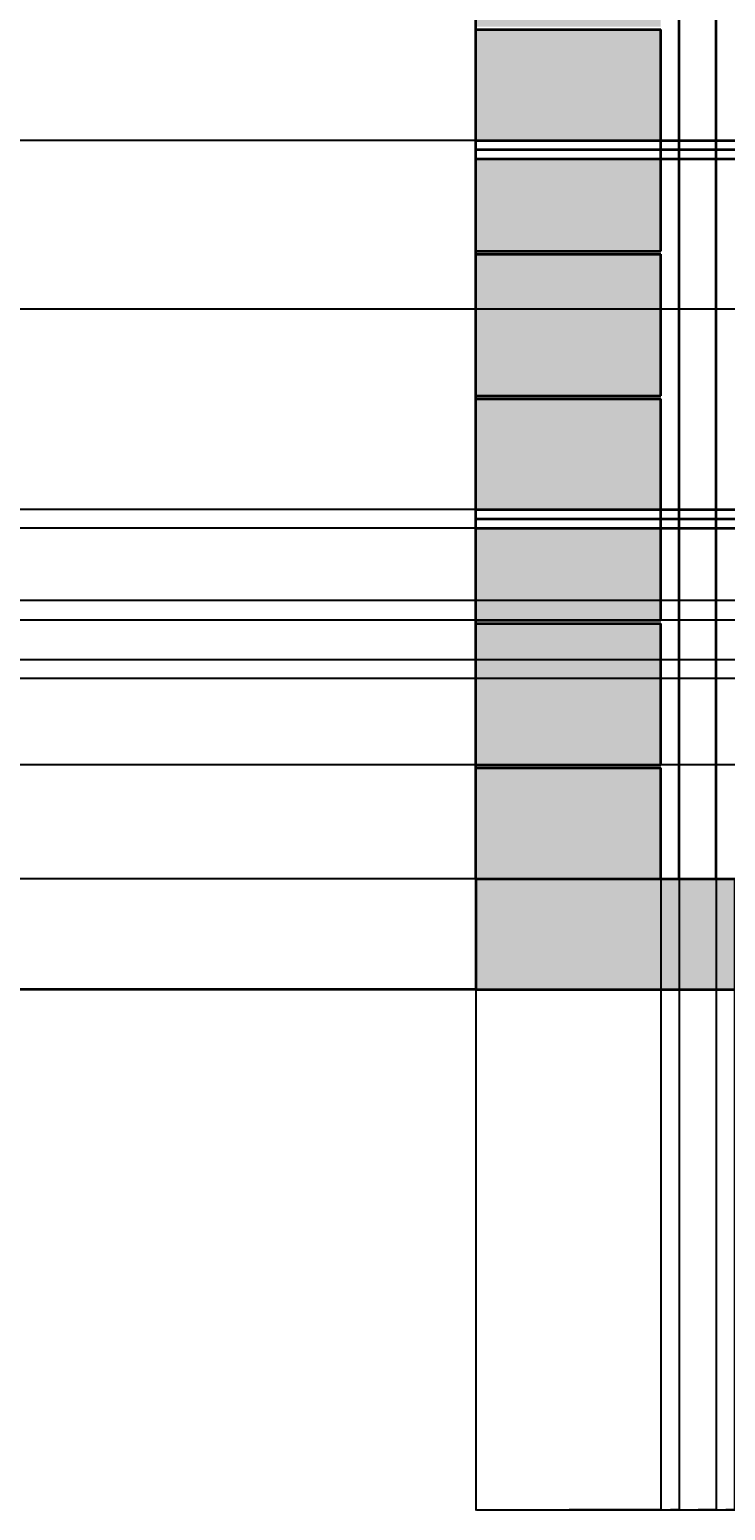
# Model space of a CAD drawing. Units: inches. Extents: x -742 to 1386, y -64 to 951.
# Tile 2 of 8: x -183 to 43, y -64 to 418. Entities that reach past the tile are written whole.
import ezdxf

# ---------------------------------------------------------------- set-up
doc = ezdxf.new("R2010")
doc.units = ezdxf.units.IN
doc.header["$MEASUREMENT"] = 0
for name, color, linetype, lineweight in [('A-ANNO-DIMS', 2, 'Continuous', 18), ('A-ELEV', 7, 'Continuous', 35), ('A-WALL-PATT', 8, 'Continuous', 13)]:
    doc.layers.add(name, color=color, linetype=linetype, lineweight=lineweight)
doc.styles.get("Standard").update_dxf_attribs({"font": 'arial.ttf'})
doc.dimstyles.get("Standard").update_dxf_attribs({"dimtxt": 0.18, "dimasz": 0.18, "dimexe": 0.18, "dimexo": 0.0625, "dimgap": 0.09, "dimtad": 0, "dimtih": 1, "dimtoh": 1, "dimdec": 4, "dimzin": 0, "dimdsep": 46, "dimtxsty": 'Standard', "dimcen": 0.09, "dimadec": 0, "dimazin": 0, "dimtfac": 1, "dimtdec": 4, "dimtofl": 0, "dimtmove": 0, "dimatfit": 3, "dimfxl": 1, "dimtolj": 1, "dimtzin": 0, "dimarcsym": 0})

# ---------------------------------------------------------------- blocks, each defined once
blk = doc.blocks.new('*D14')
at = {"layer": 'A-ANNO-DIMS', "color": 0, "lineweight": -2, "transparency": 16777216}
for p, q in [((-37.77, 105.68), (-37.77, -63.58)), ((262.23, 105.68), (262.23, -63.58)), ((-37.59, -63.4), (111.94, -63.4)), ((262.05, -63.4), (112.52, -63.4))]:
    blk.add_line(p, q, dxfattribs=at)
at = {"layer": 'A-ANNO-DIMS', "color": 0, "transparency": 16777216}
for points in [[(-37.59, -63.37), (-37.59, -63.43), (-37.77, -63.4)], [(262.05, -63.37), (262.05, -63.43), (262.23, -63.4)]]:
    blk.add_solid(points, dxfattribs=at)
at = {"layer": 'Defpoints', "color": 0, "transparency": 16777216}
for p in [(-37.77, 105.74), (262.23, 105.74), (262.23, -63.4)]:
    blk.add_point(p, dxfattribs=at)
at = {"layer": 'A-ANNO-DIMS', "color": 0, "transparency": 16777216, "insert": (112.23, -63.4), "char_height": 0.18, "attachment_point": 5}
blk.add_mtext('\\A1;300', dxfattribs=at)
blk = doc.blocks.new('*D17')
at = {"layer": 'A-ANNO-DIMS', "color": 0, "lineweight": -2, "transparency": 16777216}
for p, q in [((-37.77, 141.68), (-37.77, -63.58)), ((22.23, 141.68), (22.23, -63.58)), ((-37.59, -63.4), (-7.99, -63.4)), ((22.05, -63.4), (-7.55, -63.4))]:
    blk.add_line(p, q, dxfattribs=at)
at = {"layer": 'A-ANNO-DIMS', "color": 0, "transparency": 16777216}
for points in [[(-37.59, -63.37), (-37.59, -63.43), (-37.77, -63.4)], [(22.05, -63.37), (22.05, -63.43), (22.23, -63.4)]]:
    blk.add_solid(points, dxfattribs=at)
at = {"layer": 'Defpoints', "color": 0, "transparency": 16777216}
for p in [(-37.77, 141.74), (22.23, 141.74), (22.23, -63.4)]:
    blk.add_point(p, dxfattribs=at)
at = {"layer": 'A-ANNO-DIMS', "color": 0, "transparency": 16777216, "insert": (-7.77, -63.4), "char_height": 0.18, "attachment_point": 5}
blk.add_mtext('\\A1;60', dxfattribs=at)
blk = doc.blocks.new('*D18')
at = {"layer": 'A-ANNO-DIMS', "color": 0, "lineweight": -2, "transparency": 16777216}
for p, q in [((22.23, 141.68), (22.23, -63.58)), ((28.23, 141.68), (28.23, -63.58)), ((22.41, -63.4), (25.08, -63.4)), ((28.05, -63.4), (25.38, -63.4))]:
    blk.add_line(p, q, dxfattribs=at)
at = {"layer": 'A-ANNO-DIMS', "color": 0, "transparency": 16777216}
for points in [[(22.41, -63.37), (22.41, -63.43), (22.23, -63.4)], [(28.05, -63.37), (28.05, -63.43), (28.23, -63.4)]]:
    blk.add_solid(points, dxfattribs=at)
at = {"layer": 'Defpoints', "color": 0, "transparency": 16777216}
for p in [(22.23, 141.74), (28.23, 141.74), (28.23, -63.4)]:
    blk.add_point(p, dxfattribs=at)
at = {"layer": 'A-ANNO-DIMS', "color": 0, "transparency": 16777216, "insert": (25.23, -63.4), "char_height": 0.18, "attachment_point": 5}
blk.add_mtext('\\A1;6', dxfattribs=at)
blk = doc.blocks.new('*D19')
at = {"layer": 'A-ANNO-DIMS', "color": 0, "lineweight": -2, "transparency": 16777216}
for p, q in [((28.23, 141.68), (28.23, -63.58)), ((40.23, 141.68), (40.23, -63.58)), ((28.41, -63.4), (34.02, -63.4)), ((40.05, -63.4), (34.44, -63.4))]:
    blk.add_line(p, q, dxfattribs=at)
at = {"layer": 'A-ANNO-DIMS', "color": 0, "transparency": 16777216}
for points in [[(28.41, -63.37), (28.41, -63.43), (28.23, -63.4)], [(40.05, -63.37), (40.05, -63.43), (40.23, -63.4)]]:
    blk.add_solid(points, dxfattribs=at)
at = {"layer": 'Defpoints', "color": 0, "transparency": 16777216}
for p in [(28.23, 141.74), (40.23, 141.74), (40.23, -63.4)]:
    blk.add_point(p, dxfattribs=at)
at = {"layer": 'A-ANNO-DIMS', "color": 0, "transparency": 16777216, "insert": (34.23, -63.4), "char_height": 0.18, "attachment_point": 5}
blk.add_mtext('\\A1;12', dxfattribs=at)
blk = doc.blocks.new('*D20')
at = {"layer": 'A-ANNO-DIMS', "color": 0, "lineweight": -2, "transparency": 16777216}
for p, q in [((40.23, 141.68), (40.23, -63.58)), ((46.23, 141.68), (46.23, -63.58)), ((40.41, -63.4), (43.08, -63.4)), ((46.05, -63.4), (43.38, -63.4))]:
    blk.add_line(p, q, dxfattribs=at)
at = {"layer": 'A-ANNO-DIMS', "color": 0, "transparency": 16777216}
for points in [[(40.41, -63.37), (40.41, -63.43), (40.23, -63.4)], [(46.05, -63.37), (46.05, -63.43), (46.23, -63.4)]]:
    blk.add_solid(points, dxfattribs=at)
at = {"layer": 'Defpoints', "color": 0, "transparency": 16777216}
for p in [(40.23, 141.74), (46.23, 141.74), (46.23, -63.4)]:
    blk.add_point(p, dxfattribs=at)
at = {"layer": 'A-ANNO-DIMS', "color": 0, "transparency": 16777216, "insert": (43.23, -63.4), "char_height": 0.18, "attachment_point": 5}
blk.add_mtext('\\A1;6', dxfattribs=at)
blk = doc.blocks.new('*D40')
at = {"layer": 'A-ANNO-DIMS', "color": 0, "lineweight": -2, "transparency": 16777216}
for p, q in [((-46.83, 756.74), (-741.55, 756.74)), ((-741.37, 756.56), (-741.37, 431.42)), ((-741.37, 105.92), (-741.37, 431.06)), ((-37.83, 105.74), (-741.55, 105.74))]:
    blk.add_line(p, q, dxfattribs=at)
at = {"layer": 'A-ANNO-DIMS', "color": 0, "transparency": 16777216}
for points in [[(-741.4, 756.56), (-741.34, 756.56), (-741.37, 756.74)], [(-741.4, 105.92), (-741.34, 105.92), (-741.37, 105.74)]]:
    blk.add_solid(points, dxfattribs=at)
at = {"layer": 'Defpoints', "color": 0, "transparency": 16777216}
for p in [(-46.77, 756.74), (-741.37, 105.74), (-37.77, 105.74)]:
    blk.add_point(p, dxfattribs=at)
at = {"layer": 'A-ANNO-DIMS', "color": 0, "transparency": 16777216, "insert": (-741.37, 431.24), "char_height": 0.18, "attachment_point": 5}
blk.add_mtext('\\A1;651', dxfattribs=at)
blk = doc.blocks.new('*D41')
at = {"layer": 'A-ANNO-DIMS', "color": 0, "lineweight": -2, "transparency": 16777216}
for p, q in [((-37.83, 141.74), (-741.55, 141.74)), ((-741.37, 141.56), (-741.37, 123.92)), ((-741.37, 105.92), (-741.37, 123.56)), ((-37.83, 105.74), (-741.55, 105.74))]:
    blk.add_line(p, q, dxfattribs=at)
at = {"layer": 'A-ANNO-DIMS', "color": 0, "transparency": 16777216}
for points in [[(-741.4, 141.56), (-741.34, 141.56), (-741.37, 141.74)], [(-741.4, 105.92), (-741.34, 105.92), (-741.37, 105.74)]]:
    blk.add_solid(points, dxfattribs=at)
at = {"layer": 'Defpoints', "color": 0, "transparency": 16777216}
for p in [(-741.37, 141.74), (-37.77, 141.74), (-37.77, 105.74)]:
    blk.add_point(p, dxfattribs=at)
at = {"layer": 'A-ANNO-DIMS', "color": 0, "transparency": 16777216, "insert": (-741.37, 123.74), "char_height": 0.18, "attachment_point": 5}
blk.add_mtext('\\A1;36', dxfattribs=at)
blk = doc.blocks.new('*D42')
at = {"layer": 'A-ANNO-DIMS', "color": 0, "lineweight": -2, "transparency": 16777216}
for p, q in [((-37.83, 255.74), (-741.55, 255.74)), ((-741.37, 255.56), (-741.37, 198.92)), ((-741.37, 141.92), (-741.37, 198.56)), ((-37.83, 141.74), (-741.55, 141.74))]:
    blk.add_line(p, q, dxfattribs=at)
at = {"layer": 'A-ANNO-DIMS', "color": 0, "transparency": 16777216}
for points in [[(-741.4, 255.56), (-741.34, 255.56), (-741.37, 255.74)], [(-741.4, 141.92), (-741.34, 141.92), (-741.37, 141.74)]]:
    blk.add_solid(points, dxfattribs=at)
at = {"layer": 'Defpoints', "color": 0, "transparency": 16777216}
for p in [(-741.37, 255.74), (-37.77, 255.74), (-37.77, 141.74)]:
    blk.add_point(p, dxfattribs=at)
at = {"layer": 'A-ANNO-DIMS', "color": 0, "transparency": 16777216, "insert": (-741.37, 198.74), "char_height": 0.18, "attachment_point": 5}
blk.add_mtext('\\A1;114', dxfattribs=at)
blk = doc.blocks.new('*D43')
at = {"layer": 'A-ANNO-DIMS', "color": 0, "lineweight": -2, "transparency": 16777216}
for p, q in [((-37.83, 261.74), (-741.55, 261.74)), ((-741.37, 261.56), (-741.37, 258.92)), ((-37.83, 255.74), (-741.55, 255.74)), ((-741.37, 255.92), (-741.37, 258.56))]:
    blk.add_line(p, q, dxfattribs=at)
at = {"layer": 'A-ANNO-DIMS', "color": 0, "transparency": 16777216}
for points in [[(-741.4, 261.56), (-741.34, 261.56), (-741.37, 261.74)], [(-741.4, 255.92), (-741.34, 255.92), (-741.37, 255.74)]]:
    blk.add_solid(points, dxfattribs=at)
at = {"layer": 'Defpoints', "color": 0, "transparency": 16777216}
for p in [(-741.37, 261.74), (-37.77, 261.74), (-37.77, 255.74)]:
    blk.add_point(p, dxfattribs=at)
at = {"layer": 'A-ANNO-DIMS', "color": 0, "transparency": 16777216, "insert": (-741.37, 258.74), "char_height": 0.18, "attachment_point": 5}
blk.add_mtext('\\A1;6', dxfattribs=at)
blk = doc.blocks.new('*D44')
at = {"layer": 'A-ANNO-DIMS', "color": 0, "lineweight": -2, "transparency": 16777216}
for p, q in [((-37.83, 381.74), (-741.55, 381.74)), ((-741.37, 381.56), (-741.37, 321.92)), ((-741.37, 261.92), (-741.37, 321.56)), ((-37.83, 261.74), (-741.55, 261.74))]:
    blk.add_line(p, q, dxfattribs=at)
at = {"layer": 'A-ANNO-DIMS', "color": 0, "transparency": 16777216}
for points in [[(-741.4, 381.56), (-741.34, 381.56), (-741.37, 381.74)], [(-741.4, 261.92), (-741.34, 261.92), (-741.37, 261.74)]]:
    blk.add_solid(points, dxfattribs=at)
at = {"layer": 'Defpoints', "color": 0, "transparency": 16777216}
for p in [(-741.37, 381.74), (-37.77, 381.74), (-37.77, 261.74)]:
    blk.add_point(p, dxfattribs=at)
at = {"layer": 'A-ANNO-DIMS', "color": 0, "transparency": 16777216, "insert": (-741.37, 321.74), "char_height": 0.18, "attachment_point": 5}
blk.add_mtext('\\A1;120', dxfattribs=at)
blk = doc.blocks.new('*D45')
at = {"layer": 'A-ANNO-DIMS', "color": 0, "lineweight": -2, "transparency": 16777216}
for p, q in [((-37.83, 501.74), (-741.55, 501.74)), ((-741.37, 501.56), (-741.37, 441.92)), ((-741.37, 381.92), (-741.37, 441.56)), ((-37.83, 381.74), (-741.55, 381.74))]:
    blk.add_line(p, q, dxfattribs=at)
at = {"layer": 'A-ANNO-DIMS', "color": 0, "transparency": 16777216}
for points in [[(-741.4, 501.56), (-741.34, 501.56), (-741.37, 501.74)], [(-741.4, 381.92), (-741.34, 381.92), (-741.37, 381.74)]]:
    blk.add_solid(points, dxfattribs=at)
at = {"layer": 'Defpoints', "color": 0, "transparency": 16777216}
for p in [(-741.37, 501.74), (-37.77, 501.74), (-37.77, 381.74)]:
    blk.add_point(p, dxfattribs=at)
at = {"layer": 'A-ANNO-DIMS', "color": 0, "transparency": 16777216, "insert": (-741.37, 441.74), "char_height": 0.18, "attachment_point": 5}
blk.add_mtext('\\A1;120', dxfattribs=at)
blk = doc.blocks.new('*D49')
at = {"layer": 'A-ANNO-DIMS', "color": 0, "lineweight": -2, "transparency": 16777216}
for p, q in [((93.05, 178.74), (-741.55, 178.74)), ((-741.37, 178.56), (-741.37, 160.42)), ((-741.37, 141.92), (-741.37, 160.06)), ((46.17, 141.74), (-741.55, 141.74))]:
    blk.add_line(p, q, dxfattribs=at)
at = {"layer": 'A-ANNO-DIMS', "color": 0, "transparency": 16777216}
for points in [[(-741.4, 178.56), (-741.34, 178.56), (-741.37, 178.74)], [(-741.4, 141.92), (-741.34, 141.92), (-741.37, 141.74)]]:
    blk.add_solid(points, dxfattribs=at)
at = {"layer": 'Defpoints', "color": 0, "transparency": 16777216}
for p in [(93.11, 178.74), (-741.37, 141.74), (46.23, 141.74)]:
    blk.add_point(p, dxfattribs=at)
at = {"layer": 'A-ANNO-DIMS', "color": 0, "transparency": 16777216, "insert": (-741.37, 160.24), "char_height": 0.18, "attachment_point": 5}
blk.add_mtext('\\A1;37', dxfattribs=at)
blk = doc.blocks.new('*D50')
at = {"layer": 'A-ANNO-DIMS', "color": 0, "lineweight": -2, "transparency": 16777216}
for p, q in [((84.36, 232.23), (-741.55, 232.23)), ((-741.37, 232.05), (-741.37, 229.16)), ((-741.37, 225.92), (-741.37, 228.8)), ((93.05, 225.74), (-741.55, 225.74))]:
    blk.add_line(p, q, dxfattribs=at)
at = {"layer": 'A-ANNO-DIMS', "color": 0, "transparency": 16777216}
for points in [[(-741.4, 232.05), (-741.34, 232.05), (-741.37, 232.23)], [(-741.4, 225.92), (-741.34, 225.92), (-741.37, 225.74)]]:
    blk.add_solid(points, dxfattribs=at)
at = {"layer": 'Defpoints', "color": 0, "transparency": 16777216}
for p in [(-741.37, 232.23), (84.43, 232.23), (93.11, 225.74)]:
    blk.add_point(p, dxfattribs=at)
at = {"layer": 'A-ANNO-DIMS', "color": 0, "transparency": 16777216, "insert": (-741.37, 228.98), "char_height": 0.18, "attachment_point": 5}
blk.add_mtext('\\A1;6.486', dxfattribs=at)
blk = doc.blocks.new('*D55')
at = {"layer": 'A-ANNO-DIMS', "color": 0, "lineweight": -2, "transparency": 16777216}
for p, q in [((295.5, 326.85), (-741.55, 326.85)), ((-741.37, 326.67), (-741.37, 270.04)), ((-741.37, 213.03), (-741.37, 269.67)), ((295.5, 212.85), (-741.55, 212.85))]:
    blk.add_line(p, q, dxfattribs=at)
at = {"layer": 'A-ANNO-DIMS', "color": 0, "transparency": 16777216}
for points in [[(-741.4, 326.67), (-741.34, 326.67), (-741.37, 326.85)], [(-741.4, 213.03), (-741.34, 213.03), (-741.37, 212.85)]]:
    blk.add_solid(points, dxfattribs=at)
at = {"layer": 'Defpoints', "color": 0, "transparency": 16777216}
for p in [(-741.37, 326.85), (295.56, 326.85), (295.56, 212.85)]:
    blk.add_point(p, dxfattribs=at)
at = {"layer": 'A-ANNO-DIMS', "color": 0, "transparency": 16777216, "insert": (-741.37, 269.85), "char_height": 0.18, "attachment_point": 5}
blk.add_mtext('\\A1;114', dxfattribs=at)
blk = doc.blocks.new('*D56')
at = {"layer": 'A-ANNO-DIMS', "color": 0, "lineweight": -2, "transparency": 16777216}
for p, q in [((268.17, 212.85), (-741.55, 212.85)), ((-741.37, 212.67), (-741.37, 210.04)), ((-741.37, 207.03), (-741.37, 209.67)), ((268.17, 206.85), (-741.55, 206.85))]:
    blk.add_line(p, q, dxfattribs=at)
at = {"layer": 'A-ANNO-DIMS', "color": 0, "transparency": 16777216}
for points in [[(-741.4, 212.67), (-741.34, 212.67), (-741.37, 212.85)], [(-741.4, 207.03), (-741.34, 207.03), (-741.37, 206.85)]]:
    blk.add_solid(points, dxfattribs=at)
at = {"layer": 'Defpoints', "color": 0, "transparency": 16777216}
for p in [(-741.37, 212.85), (268.23, 212.85), (268.23, 206.85)]:
    blk.add_point(p, dxfattribs=at)
at = {"layer": 'A-ANNO-DIMS', "color": 0, "transparency": 16777216, "insert": (-741.37, 209.85), "char_height": 0.18, "attachment_point": 5}
blk.add_mtext('\\A1;6', dxfattribs=at)

msp = doc.modelspace()

# ---------------------------------------------------------------- hatches: boundary and pattern name
at = {"layer": 'A-WALL-PATT', "transparency": 33554457}
h = msp.add_hatch(dxfattribs=at)
h.set_pattern_fill('AR-B88', color=256)
h.paths.add_polyline_path([(22.2276, 224.7399), (-37.7724, 224.7399), (-37.7724, 178.7399), (22.2276, 178.7399)])
h.paths.add_polyline_path([(22.2276, 177.7399), (-37.7724, 177.7399), (-37.7724, 141.7399), (22.2276, 141.7399)])
h.paths.add_polyline_path([(22.2276, 255.7399), (-37.7724, 255.7399), (-37.7724, 225.7399), (22.2276, 225.7399)])
h.paths.add_polyline_path([(22.2276, 297.7399), (-37.7724, 297.7399), (-37.7724, 261.7399), (22.2276, 261.7399)])
h.paths.add_polyline_path([(22.2276, 344.7399), (-37.7724, 344.7399), (-37.7724, 298.7399), (22.2276, 298.7399)])
h.paths.add_polyline_path([(22.2276, 375.7399), (-37.7724, 375.7399), (-37.7724, 345.7399), (22.2276, 345.7399)])
h.paths.add_polyline_path([(22.2276, 417.7399), (-37.7724, 417.7399), (-37.7724, 381.7399), (22.2276, 381.7399)])
h.paths.add_polyline_path([(22.2276, 464.7399), (-37.7724, 464.7399), (-37.7724, 418.7399), (22.2276, 418.7399)])
h.paths.add_polyline_path([(22.2276, 495.7399), (-37.7724, 495.7399), (-37.7724, 465.7399), (22.2276, 465.7399)])
h.paths.add_polyline_path([(22.2276, 537.7399), (-37.7724, 537.7399), (-37.7724, 501.7399), (22.2276, 501.7399)])
h.paths.add_polyline_path([(22.2276, 584.7399), (-37.7724, 584.7399), (-37.7724, 538.7399), (22.2276, 538.7399)])
h.paths.add_polyline_path([(22.2276, 615.7399), (-37.7724, 615.7399), (-37.7724, 585.7399), (22.2276, 585.7399)])
h.paths.add_polyline_path([(22.2276, 657.7399), (-37.7724, 657.7399), (-37.7724, 621.7399), (22.2276, 621.7399)])
h.paths.add_polyline_path([(22.2276, 704.7399), (-37.7724, 704.7399), (-37.7724, 658.7399), (22.2276, 658.7399)])
h.paths.add_polyline_path([(22.2276, 735.7399), (-37.7724, 735.7399), (-37.7724, 705.7399), (22.2276, 705.7399)])
h.paths.add_polyline_path([(376.2276, 835.7799), (268.2276, 835.7799), (268.2276, 806.8548), (376.2276, 806.8548)])
h.paths.add_polyline_path([(682.2276, 735.7399), (622.2276, 735.7399), (622.2276, 705.7399), (682.2276, 705.7399)])
h.paths.add_polyline_path([(682.2276, 704.7399), (622.2276, 704.7399), (622.2276, 658.7399), (682.2276, 658.7399)])
h.paths.add_polyline_path([(682.2276, 657.7399), (622.2276, 657.7399), (622.2276, 621.7399), (682.2276, 621.7399)])
h.paths.add_polyline_path([(682.2276, 615.7399), (622.2276, 615.7399), (622.2276, 585.7399), (682.2276, 585.7399)])
h.paths.add_polyline_path([(682.2276, 584.7399), (622.2276, 584.7399), (622.2276, 538.7399), (682.2276, 538.7399)])
h.paths.add_polyline_path([(682.2276, 537.7399), (622.2276, 537.7399), (622.2276, 501.7399), (682.2276, 501.7399)])
h.paths.add_polyline_path([(682.2276, 495.7399), (622.2276, 495.7399), (622.2276, 465.7399), (682.2276, 465.7399)])
h.paths.add_polyline_path([(682.2276, 464.7399), (622.2276, 464.7399), (622.2276, 418.7399), (682.2276, 418.7399)])
h.paths.add_polyline_path([(682.2276, 417.7399), (622.2276, 417.7399), (622.2276, 381.7399), (682.2276, 381.7399)])
h.paths.add_polyline_path([(682.2276, 375.7399), (622.2276, 375.7399), (622.2276, 345.7399), (682.2276, 345.7399)])
h.paths.add_polyline_path([(682.2276, 344.7399), (622.2276, 344.7399), (622.2276, 298.7399), (682.2276, 298.7399)])
h.paths.add_polyline_path([(682.2276, 297.7399), (622.2276, 297.7399), (622.2276, 261.7399), (682.2276, 261.7399)])
h.paths.add_polyline_path([(682.2276, 255.7399), (622.2276, 255.7399), (622.2276, 225.7399), (682.2276, 225.7399)])
h.paths.add_polyline_path([(682.2276, 224.7399), (622.2276, 224.7399), (622.2276, 178.7399), (682.2276, 178.7399)])
h.paths.add_polyline_path([(682.2276, 177.7399), (622.2276, 177.7399), (622.2276, 141.7399), (682.2276, 141.7399)])
h = msp.add_hatch(dxfattribs=at)
h.set_pattern_fill('GRAVEL', color=256, scale=40)
h.paths.add_polyline_path([(262.2276, 141.7399), (-37.7724, 141.7399), (-37.7724, 105.7399), (262.2276, 105.7399)])
h.paths.add_polyline_path([(682.2276, 141.7399), (382.2276, 141.7399), (382.2276, 105.7399), (682.2276, 105.7399)])

# ---------------------------------------------------------------- linework, layer by layer
at = {"layer": 'A-ELEV'}
for p, q in [((-37.7724, 141.7399), (-37.7724, 741.7399)), ((28.2276, 141.7399), (28.2276, 741.7399)), ((40.2276, 141.7399), (40.2276, 741.7399)), ((-37.7724, 417.7399), (22.2276, 417.7399)), ((22.2276, 345.7399), (22.2276, 417.7399)), ((-37.7724, 381.7399), (268.2276, 381.7399)), ((-37.7724, 378.7399), (268.2276, 378.7399)), ((-37.7724, 375.7399), (268.2276, 375.7399)), ((-37.7724, 345.7399), (22.2276, 345.7399)), ((-37.7724, 344.7399), (22.2276, 344.7399)), ((22.2276, 298.7399), (22.2276, 344.7399)), ((-37.7724, 298.7399), (22.2276, 298.7399)), ((-37.7724, 297.7399), (22.2276, 297.7399)), ((22.2276, 225.7399), (22.2276, 297.7399)), ((-37.7724, 261.7399), (268.2276, 261.7399)), ((-37.7724, 258.7399), (268.2276, 258.7399)), ((-37.7724, 255.7399), (268.2276, 255.7399)), ((-37.7724, 225.7399), (22.2276, 225.7399)), ((-37.7724, 224.7399), (22.2276, 224.7399)), ((22.2276, 178.7399), (22.2276, 224.7399)), ((-37.7724, 178.7399), (22.2276, 178.7399)), ((-37.7724, 177.7399), (22.2276, 177.7399)), ((22.2276, 141.7399), (22.2276, 177.7399)), ((-37.7724, 141.7399), (262.2276, 141.7399)), ((-37.7724, 141.7399), (-37.7724, 105.7399)), ((-37.7724, 105.7399), (-644.1211, 105.7399)), ((-37.7724, 105.7399), (262.2276, 105.7399))]:
    msp.add_line(p, q, dxfattribs=at)

# ---------------------------------------------------------------- dimensions: what is measured, and where the dimension line sits
at = {"layer": 'A-ANNO-DIMS'}
for base, p1, p2, override, picture, middle in [((-741.3711, 105.7399), (-46.7724, 756.7399), (-37.7724, 105.7399), {"dimdec": 0, "dimlfac": 1, "dimrnd": 0, "dimzin": 0, "dimdsep": 46, "dimlunit": 2}, '*D40', (-741.3711, 431.2399)), ((-741.3711, 501.7399), (-37.7724, 381.7399), (-37.7724, 501.7399), {"dimdec": 0, "dimlfac": 1, "dimrnd": 0, "dimzin": 0, "dimdsep": 46, "dimlunit": 2}, '*D45', (-741.3711, 441.7399)), ((-741.3711, 381.7399), (-37.7724, 261.7399), (-37.7724, 381.7399), {"dimdec": 0, "dimlfac": 1, "dimrnd": 0, "dimzin": 0, "dimdsep": 46, "dimlunit": 2}, '*D44', (-741.3711, 321.7399)), ((-741.3711, 326.8548), (295.5643, 212.8548), (295.5643, 326.8548), {"dimdec": 0, "dimlfac": 1, "dimrnd": 0, "dimzin": 0, "dimdsep": 46, "dimlunit": 2}, '*D55', (-741.3711, 269.8548)), ((-741.3711, 261.7399), (-37.7724, 255.7399), (-37.7724, 261.7399), {"dimdec": 0, "dimlfac": 1, "dimrnd": 0, "dimzin": 0, "dimdsep": 46, "dimlunit": 2}, '*D43', (-741.3711, 258.7399)), ((-741.3711, 255.7399), (-37.7724, 141.7399), (-37.7724, 255.7399), {"dimdec": 0, "dimlfac": 1, "dimrnd": 0, "dimzin": 0, "dimdsep": 46, "dimlunit": 2}, '*D42', (-741.3711, 198.7399)), ((-741.37107, 232.22544), (93.11175, 225.73986), (84.42625, 232.22544), {"dimdec": 3, "dimlfac": 1, "dimrnd": 0, "dimzin": 0, "dimdsep": 46, "dimlunit": 2}, '*D50', (-741.37107, 228.98265)), ((-741.3711, 212.8548), (268.2276, 206.8548), (268.2276, 212.8548), {"dimdec": 0, "dimlfac": 1, "dimrnd": 0, "dimzin": 0, "dimdsep": 46, "dimlunit": 2}, '*D56', (-741.3711, 209.8548)), ((-741.3711, 141.7399), (93.1117, 178.7399), (46.2276, 141.7399), {"dimdec": 0, "dimlfac": 1, "dimrnd": 0, "dimzin": 0, "dimdsep": 46, "dimlunit": 2}, '*D49', (-741.3711, 160.2399)), ((-741.3711, 141.7399), (-37.7724, 105.7399), (-37.7724, 141.7399), {"dimdec": 0, "dimlfac": 1, "dimrnd": 0, "dimzin": 0, "dimdsep": 46, "dimlunit": 2}, '*D41', (-741.3711, 123.7399))]:
    dim = msp.add_linear_dim(base=base, p1=p1, p2=p2, angle=90, dimstyle='Standard', override=override, dxfattribs=at)
    dim.commit()
    dim.dimension.update_dxf_attribs({"geometry": picture, "text_midpoint": middle})
for base, p1, p2, picture, middle in [((22.2276, -63.3971), (-37.7724, 141.7399), (22.2276, 141.7399), '*D17', (-7.7724, -63.3971)), ((28.2276, -63.3971), (22.2276, 141.7399), (28.2276, 141.7399), '*D18', (25.2276, -63.3971)), ((40.2276, -63.3971), (28.2276, 141.7399), (40.2276, 141.7399), '*D19', (34.2276, -63.3971)), ((46.2276, -63.3971), (40.2276, 141.7399), (46.2276, 141.7399), '*D20', (43.2276, -63.3971)), ((262.2276, -63.3971), (-37.7724, 105.7399), (262.2276, 105.7399), '*D14', (112.2276, -63.3971))]:
    dim = msp.add_linear_dim(base=base, p1=p1, p2=p2, dimstyle='Standard', override={"dimdec": 0, "dimlfac": 1, "dimrnd": 0, "dimzin": 0, "dimdsep": 46, "dimlunit": 2}, dxfattribs=at)
    dim.commit()
    dim.dimension.update_dxf_attribs({"geometry": picture, "text_midpoint": middle})

doc.saveas('drawing.dxf')
